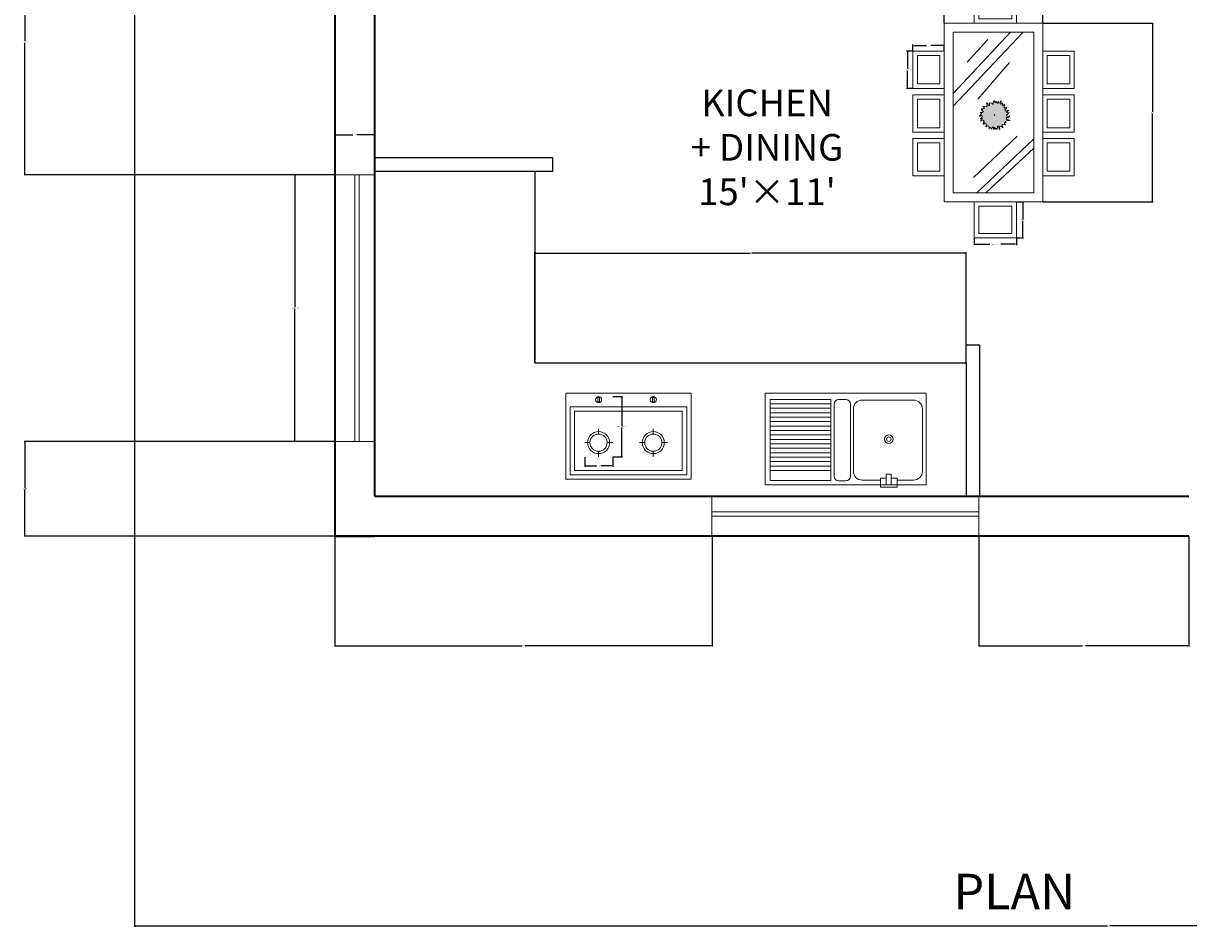
# Model space of a CAD drawing. Units: inches. Extents: x 1315 to 1802, y 1702 to 2202.
# Tile 1 of 4: x 1315 to 1577, y 1702 to 1906. Entities that reach past the tile are written whole.
import ezdxf

# ---------------------------------------------------------------- set-up
doc = ezdxf.new("R2010")
doc.units = ezdxf.units.IN
for name, color, linetype, lineweight in [('A-ANNO-DIMS', 2, 'Continuous', 18), ('A-ANNO-TEXT', 3, 'Continuous', 25), ('A-AREA-IDEN', 3, 'Continuous', 18), ('A-CASE', 7, 'Continuous', 25), ('A-EQPM', 3, 'Continuous', 18), ('A-FLOR-FIXT', 30, 'Continuous', 18), ('A-FLOR-FIXT-PATT', 30, 'Continuous', 13), ('A-FURN', 8, 'Continuous', 18), ('A-FURN-PATT', 9, 'Continuous', 13), ('A-GLAZ', 4, 'Continuous', 18), ('A-WALL', 7, 'Continuous', 35)]:
    doc.layers.add(name, color=color, linetype=linetype, lineweight=lineweight)
doc.styles.get("Standard").update_dxf_attribs({"font": 'times.ttf'})
doc.dimstyles.get("Standard").update_dxf_attribs({"dimtxt": 0.18, "dimasz": 0.18, "dimexe": 0.18, "dimexo": 0.0625, "dimgap": 0.09, "dimtad": 0, "dimtih": 1, "dimtoh": 1, "dimdec": 4, "dimzin": 0, "dimdsep": 46, "dimtxsty": 'Standard', "dimcen": 0.09, "dimadec": 0, "dimazin": 0, "dimtfac": 1, "dimtdec": 4, "dimtofl": 0, "dimtmove": 0, "dimatfit": 3, "dimfxl": 1, "dimtolj": 1, "dimtzin": 0, "dimarcsym": 0})

# ---------------------------------------------------------------- blocks, each defined once
blk = doc.blocks.new('*U2')
for points in [[(0, 60.64), (-3.051, 56.238), (-4.196, 52.815), (-5.34, 47.925), (-6.103, 45.969), (-11.062, 50.859), (-18.691, 52.326), (-20.98, 47.436), (-20.217, 43.524), (-20.598, 39.611), (-25.939, 43.035), (-27.846, 49.392), (-33.186, 52.326), (-30.516, 47.436), (-31.279, 43.035), (-30.135, 38.144), (-33.568, 35.21), (-40.815, 36.677), (-49.208, 38.144), (-46.919, 36.677), (-42.341, 31.787), (-42.341, 28.364), (-46.537, 27.386), (-55.692, 27.386), (-49.97, 22.006), (-54.548, 21.028), (-46.156, 14.671), (-51.496, 11.248), (-59.888, 11.248), (-55.692, 8.803), (-53.785, 5.38), (-57.218, 3.423), (-60.651, -1.467), (-61.033, -4.89), (-59.125, -3.423), (-54.548, -1.467), (-51.496, -4.401), (-53.022, -10.269), (-59.125, -15.16), (-49.208, -13.204), (-58.362, -24.451), (-48.445, -21.028), (-43.486, -22.495), (-43.104, -25.918), (-47.3, -31.298), (-43.104, -30.32), (-48.445, -39.611), (-38.527, -31.787), (-40.815, -36.188), (-32.423, -37.166), (-33.568, -43.523), (-35.475, -49.392), (-28.609, -44.99), (-23.65, -46.457), (-22.124, -51.837), (-21.743, -57.705), (-19.073, -52.326), (-15.639, -51.837), (-12.588, -58.683), (-11.062, -54.771), (-6.866, -49.392), (-6.866, -53.304), (-4.959, -48.414), (-1.907, -61.617), (-1.144, -51.348), (4.578, -59.172), (5.341, -54.282), (9.918, -56.727), (12.207, -60.639), (12.97, -47.925), (14.877, -44.501), (17.547, -47.436), (19.455, -52.815), (22.888, -60.639), (21.743, -49.392), (23.65, -46.457), (29.754, -47.925), (35.094, -52.326), (37.001, -53.793), (33.187, -46.457), (32.042, -41.567), (35.094, -39.122), (43.868, -40.589), (47.682, -42.056), (43.105, -36.188), (43.105, -33.743), (46.538, -31.298), (50.352, -32.765), (46.919, -26.407), (55.693, -22.495), (60.652, -22.984), (66.374, -22.006), (59.889, -20.05), (54.167, -18.094), (51.878, -15.649), (49.589, -12.225), (51.497, -10.269), (57.981, -9.78), (63.322, -7.335), (64.466, -2.934)], [(64.848, -2.934), (59.507, -5.379), (56.456, -4.401), (51.878, -2.445), (52.26, 0.978), (55.311, 3.912), (59.889, 5.869), (62.94, 11.248), (58.363, 10.27), (54.548, 10.27), (51.115, 11.248), (53.785, 15.649), (57.981, 18.094), (60.652, 19.561), (56.074, 19.561), (51.115, 17.605), (46.538, 19.072), (46.156, 22.496), (49.589, 27.386), (52.26, 34.721), (49.589, 33.743), (44.249, 30.32), (41.197, 32.276), (41.579, 37.655), (43.868, 42.546), (43.105, 46.947), (40.053, 44.013), (36.238, 40.589), (33.568, 42.057), (33.95, 45.969), (35.476, 52.815), (31.28, 49.392), (26.702, 46.947), (28.228, 50.859), (28.609, 61.129), (24.795, 54.282), (18.692, 50.859), (17.929, 57.706), (12.97, 50.859), (7.248, 57.706), (5.341, 53.304), (0, 60.64)]]:
    blk.add_lwpolyline(points)
blk.add_lwpolyline([(0.382, 1.956), (0, 0), (1.907, 0.489), (2.289, 1.467)], close=True)
blk = doc.blocks.new('SEFVFT')
for p, q in [((1768.59, 1985.26), (1777.59, 1985.26)), ((1768.59, 1925.26), (1768.59, 1985.26)), ((1768.59, 1985.26), (1773.09, 1985.26)), ((1773.09, 1985.26), (1773.09, 1925.26)), ((1774.09, 1925.26), (1774.09, 1985.26)), ((1777.59, 1985.26), (1777.59, 1925.26)), ((1777.59, 1925.26), (1768.59, 1925.26)), ((1773.09, 1925.26), (1774.09, 1925.26))]:
    blk.add_line(p, q)
blk = doc.blocks.new('CHAIR-DINING-SIDE')
for points in [[(0, 8.39), (7.03, 8.39), (7.03, 0), (0, 0)], [(1, 7.39), (6.03, 7.39), (6.03, 1), (1, 1)]]:
    blk.add_lwpolyline(points, close=True)
blk = doc.blocks.new('CHAIR-DINING-END')
for points in [[(0, 0), (9.48, 0), (9.48, 8.13), (0, 8.13)], [(1, 1), (8.48, 1), (8.48, 7.13), (1, 7.13)]]:
    blk.add_lwpolyline(points, close=True)
blk = doc.blocks.new('COOKTOP-BURNER-CONTROL')
for p, q in [((3.08, 5.13), (3.08, 6.3)), ((3.08, 6.3), (3.08, 5.13)), ((1.15, 3.2), (0, 3.2)), ((5.01, 3.2), (6.25, 3.2)), ((6.25, 3.2), (5.01, 3.2)), ((3.08, 1.27), (3.08, 0))]:
    blk.add_line(p, q)
blk.add_lwpolyline([(2.89, 12.39), (3.26, 12.39), (3.26, 13.37), (2.89, 13.37)], close=True)
for centre, radius in [((3.08, 12.88), 0.694), ((3.08, 3.2), 2.47), ((3.08, 3.2), 1.93)]:
    blk.add_circle(centre, radius)
blk = doc.blocks.new('*D12')
at = {"layer": 'A-ANNO-DIMS', "color": 0, "lineweight": -2, "transparency": 16777216}
for p, q in [((1384.53, 1871.52), (1375.41, 1871.52)), ((1375.59, 1871.34), (1375.59, 1841.7)), ((1375.59, 1811.7), (1375.59, 1841.34)), ((1384.53, 1811.52), (1375.41, 1811.52))]:
    blk.add_line(p, q, dxfattribs=at)
at = {"layer": 'A-ANNO-DIMS', "color": 0, "transparency": 16777216}
for points in [[(1375.56, 1871.34), (1375.62, 1871.34), (1375.59, 1871.52)], [(1375.56, 1811.7), (1375.62, 1811.7), (1375.59, 1811.52)]]:
    blk.add_solid(points, dxfattribs=at)
at = {"layer": 'Defpoints', "color": 0, "transparency": 16777216}
for p in [(1375.59, 1871.52), (1384.59, 1871.52), (1384.59, 1811.52)]:
    blk.add_point(p, dxfattribs=at)
at = {"layer": 'A-ANNO-DIMS', "color": 0, "transparency": 16777216, "insert": (1375.59, 1841.52), "char_height": 0.18, "attachment_point": 5}
blk.add_mtext('\\A1;WINDOW 60 TYP.', dxfattribs=at)
blk = doc.blocks.new('*D13')
at = {"layer": 'A-ANNO-DIMS', "color": 0, "lineweight": -2, "transparency": 16777216}
for p, q in [((1384.59, 1871.58), (1384.59, 1880.7)), ((1384.77, 1880.52), (1388.63, 1880.52)), ((1393.41, 1880.52), (1389.55, 1880.52)), ((1393.59, 1871.58), (1393.59, 1880.7))]:
    blk.add_line(p, q, dxfattribs=at)
at = {"layer": 'A-ANNO-DIMS', "color": 0, "transparency": 16777216}
for points in [[(1384.77, 1880.55), (1384.77, 1880.49), (1384.59, 1880.52)], [(1393.41, 1880.55), (1393.41, 1880.49), (1393.59, 1880.52)]]:
    blk.add_solid(points, dxfattribs=at)
at = {"layer": 'Defpoints', "color": 0, "transparency": 16777216}
for p in [(1393.59, 1880.52), (1384.59, 1871.52), (1393.59, 1871.52)]:
    blk.add_point(p, dxfattribs=at)
at = {"layer": 'A-ANNO-DIMS', "color": 0, "transparency": 16777216, "insert": (1389.09, 1880.52), "char_height": 0.18, "attachment_point": 5}
blk.add_mtext('\\A1;9 TYP.', dxfattribs=at)
blk = doc.blocks.new('*D18')
at = {"layer": 'A-ANNO-DIMS', "color": 0, "lineweight": -2, "transparency": 16777216}
for p, q in [((1514.54, 1899.33), (1513.16, 1899.33)), ((1513.34, 1899.15), (1513.34, 1895.32)), ((1513.34, 1891.12), (1513.34, 1894.95)), ((1514.54, 1890.94), (1513.16, 1890.94))]:
    blk.add_line(p, q, dxfattribs=at)
at = {"layer": 'A-ANNO-DIMS', "color": 0, "transparency": 16777216}
for points in [[(1513.31, 1899.15), (1513.37, 1899.15), (1513.34, 1899.33)], [(1513.31, 1891.12), (1513.37, 1891.12), (1513.34, 1890.94)]]:
    blk.add_solid(points, dxfattribs=at)
at = {"layer": 'Defpoints', "color": 0, "transparency": 16777216}
for p in [(1513.34, 1899.33), (1514.6, 1899.33), (1514.6, 1890.94)]:
    blk.add_point(p, dxfattribs=at)
at = {"layer": 'A-ANNO-DIMS', "color": 0, "transparency": 16777216, "insert": (1513.34, 1895.14), "char_height": 0.18, "attachment_point": 5}
blk.add_mtext('\\A1;SIDE CHAIR 8 TYP.', dxfattribs=at)
blk = doc.blocks.new('*D19')
at = {"layer": 'A-ANNO-DIMS', "color": 0, "lineweight": -2, "transparency": 16777216}
for p, q in [((1514.6, 1899.39), (1514.6, 1900.77)), ((1514.78, 1900.59), (1517.66, 1900.59)), ((1521.46, 1900.59), (1518.58, 1900.59)), ((1521.64, 1899.39), (1521.64, 1900.77))]:
    blk.add_line(p, q, dxfattribs=at)
at = {"layer": 'A-ANNO-DIMS', "color": 0, "transparency": 16777216}
for points in [[(1514.78, 1900.62), (1514.78, 1900.56), (1514.6, 1900.59)], [(1521.46, 1900.62), (1521.46, 1900.56), (1521.64, 1900.59)]]:
    blk.add_solid(points, dxfattribs=at)
at = {"layer": 'Defpoints', "color": 0, "transparency": 16777216}
for p in [(1521.64, 1900.59), (1514.6, 1899.33), (1521.64, 1899.33)]:
    blk.add_point(p, dxfattribs=at)
at = {"layer": 'A-ANNO-DIMS', "color": 0, "transparency": 16777216, "insert": (1518.12, 1900.59), "char_height": 0.18, "attachment_point": 5}
blk.add_mtext('\\A1;7 TYP.', dxfattribs=at)
blk = doc.blocks.new('*D20')
at = {"layer": 'A-ANNO-DIMS', "color": 0, "lineweight": -2, "transparency": 16777216}
for p, q in [((1528.38, 1857.23), (1528.38, 1855.69)), ((1528.56, 1855.87), (1531.91, 1855.87)), ((1537.68, 1855.87), (1534.34, 1855.87)), ((1537.86, 1857.23), (1537.86, 1855.69))]:
    blk.add_line(p, q, dxfattribs=at)
at = {"layer": 'A-ANNO-DIMS', "color": 0, "transparency": 16777216}
for points in [[(1528.56, 1855.9), (1528.56, 1855.84), (1528.38, 1855.87)], [(1537.68, 1855.9), (1537.68, 1855.84), (1537.86, 1855.87)]]:
    blk.add_solid(points, dxfattribs=at)
at = {"layer": 'Defpoints', "color": 0, "transparency": 16777216}
for p in [(1528.38, 1857.3), (1537.86, 1857.3), (1537.86, 1855.87)]:
    blk.add_point(p, dxfattribs=at)
at = {"layer": 'A-ANNO-DIMS', "color": 0, "transparency": 16777216, "insert": (1533.12, 1855.87), "char_height": 0.18, "attachment_point": 5}
blk.add_mtext('\\A1;END CHAIR 9 TYP.', dxfattribs=at)
blk = doc.blocks.new('*D21')
at = {"layer": 'A-ANNO-DIMS', "color": 0, "lineweight": -2, "transparency": 16777216}
for p, q in [((1537.92, 1865.42), (1539.46, 1865.42)), ((1539.28, 1865.24), (1539.28, 1861.54)), ((1539.28, 1857.48), (1539.28, 1861.18)), ((1537.92, 1857.3), (1539.46, 1857.3))]:
    blk.add_line(p, q, dxfattribs=at)
at = {"layer": 'A-ANNO-DIMS', "color": 0, "transparency": 16777216}
for points in [[(1539.25, 1865.24), (1539.31, 1865.24), (1539.28, 1865.42)], [(1539.25, 1857.48), (1539.31, 1857.48), (1539.28, 1857.3)]]:
    blk.add_solid(points, dxfattribs=at)
at = {"layer": 'Defpoints', "color": 0, "transparency": 16777216}
for p in [(1537.86, 1865.42), (1539.28, 1865.42), (1537.86, 1857.3)]:
    blk.add_point(p, dxfattribs=at)
at = {"layer": 'A-ANNO-DIMS', "color": 0, "transparency": 16777216, "insert": (1539.28, 1861.36), "char_height": 0.18, "attachment_point": 5}
blk.add_mtext('\\A1;8 TYP.', dxfattribs=at)
blk = doc.blocks.new('*D22')
at = {"layer": 'A-ANNO-DIMS', "color": 0, "lineweight": -2, "transparency": 16777216}
for p, q in [((1447.14, 1821.64), (1449.29, 1821.64)), ((1449.11, 1821.46), (1449.11, 1815.04)), ((1449.11, 1808.25), (1449.11, 1814.68)), ((1447.14, 1808.07), (1449.29, 1808.07))]:
    blk.add_line(p, q, dxfattribs=at)
at = {"layer": 'A-ANNO-DIMS', "color": 0, "transparency": 16777216}
for points in [[(1449.08, 1821.46), (1449.14, 1821.46), (1449.11, 1821.64)], [(1449.08, 1808.25), (1449.14, 1808.25), (1449.11, 1808.07)]]:
    blk.add_solid(points, dxfattribs=at)
at = {"layer": 'Defpoints', "color": 0, "transparency": 16777216}
for p in [(1447.08, 1821.64), (1449.11, 1821.64), (1447.08, 1808.07)]:
    blk.add_point(p, dxfattribs=at)
at = {"layer": 'A-ANNO-DIMS', "color": 0, "transparency": 16777216, "insert": (1449.11, 1814.86), "char_height": 0.18, "attachment_point": 5}
blk.add_mtext('\\A1;BURNER UNIT 14 TYP.', dxfattribs=at)
blk = doc.blocks.new('*D23')
at = {"layer": 'A-ANNO-DIMS', "color": 0, "lineweight": -2, "transparency": 16777216}
for p, q in [((1440.83, 1808.01), (1440.83, 1805.85)), ((1447.08, 1808.01), (1447.08, 1805.85)), ((1441.01, 1806.03), (1443.49, 1806.03)), ((1446.9, 1806.03), (1444.41, 1806.03))]:
    blk.add_line(p, q, dxfattribs=at)
at = {"layer": 'A-ANNO-DIMS', "color": 0, "transparency": 16777216}
for points in [[(1441.01, 1806.06), (1441.01, 1806), (1440.83, 1806.03)], [(1446.9, 1806.06), (1446.9, 1806), (1447.08, 1806.03)]]:
    blk.add_solid(points, dxfattribs=at)
at = {"layer": 'Defpoints', "color": 0, "transparency": 16777216}
for p in [(1440.83, 1808.07), (1447.08, 1808.07), (1447.08, 1806.03)]:
    blk.add_point(p, dxfattribs=at)
at = {"layer": 'A-ANNO-DIMS', "color": 0, "transparency": 16777216, "insert": (1443.95, 1806.03), "char_height": 0.18, "attachment_point": 5}
blk.add_mtext('\\A1;6 TYP.', dxfattribs=at)
blk = doc.blocks.new('*D28')
at = {"layer": 'A-ANNO-DIMS', "color": 0, "lineweight": -2, "transparency": 16777216}
for p, q in [((1339.59, 1931.18), (1339.59, 1702.41)), ((1777.59, 1763.18), (1777.59, 1702.41)), ((1339.77, 1702.59), (1558.31, 1702.59)), ((1777.41, 1702.59), (1558.87, 1702.59))]:
    blk.add_line(p, q, dxfattribs=at)
at = {"layer": 'A-ANNO-DIMS', "color": 0, "transparency": 16777216}
for points in [[(1339.77, 1702.62), (1339.77, 1702.56), (1339.59, 1702.59)], [(1777.41, 1702.62), (1777.41, 1702.56), (1777.59, 1702.59)]]:
    blk.add_solid(points, dxfattribs=at)
at = {"layer": 'Defpoints', "color": 0, "transparency": 16777216}
for p in [(1339.59, 1931.24), (1777.59, 1763.24), (1777.59, 1702.59)]:
    blk.add_point(p, dxfattribs=at)
at = {"layer": 'A-ANNO-DIMS', "color": 0, "transparency": 16777216, "insert": (1558.59, 1702.59), "char_height": 0.18, "attachment_point": 5}
blk.add_mtext('\\A1;438', dxfattribs=at)
blk = doc.blocks.new('*D39')
at = {"layer": 'A-ANNO-DIMS', "color": 0, "lineweight": -2, "transparency": 16777216}
for p, q in [((1384.53, 1931.24), (1314.76, 1931.24)), ((1314.94, 1931.06), (1314.94, 1901.56)), ((1314.94, 1871.7), (1314.94, 1901.2)), ((1384.53, 1871.52), (1314.76, 1871.52))]:
    blk.add_line(p, q, dxfattribs=at)
at = {"layer": 'A-ANNO-DIMS', "color": 0, "transparency": 16777216}
for points in [[(1314.91, 1931.06), (1314.97, 1931.06), (1314.94, 1931.24)], [(1314.91, 1871.7), (1314.97, 1871.7), (1314.94, 1871.52)]]:
    blk.add_solid(points, dxfattribs=at)
at = {"layer": 'Defpoints', "color": 0, "transparency": 16777216}
for p in [(1384.59, 1931.24), (1314.94, 1871.52), (1384.59, 1871.52)]:
    blk.add_point(p, dxfattribs=at)
at = {"layer": 'A-ANNO-DIMS', "color": 0, "transparency": 16777216, "insert": (1314.94, 1901.38), "char_height": 0.18, "attachment_point": 5}
blk.add_mtext('\\A1;59.72', dxfattribs=at)
blk = doc.blocks.new('*D40')
at = {"layer": 'A-ANNO-DIMS', "color": 0, "lineweight": -2, "transparency": 16777216}
for p, q in [((1384.53, 1811.52), (1314.76, 1811.52)), ((1314.94, 1811.34), (1314.94, 1801.06)), ((1314.94, 1790.42), (1314.94, 1800.7)), ((1384.53, 1790.24), (1314.76, 1790.24))]:
    blk.add_line(p, q, dxfattribs=at)
at = {"layer": 'A-ANNO-DIMS', "color": 0, "transparency": 16777216}
for points in [[(1314.91, 1811.34), (1314.97, 1811.34), (1314.94, 1811.52)], [(1314.91, 1790.42), (1314.97, 1790.42), (1314.94, 1790.24)]]:
    blk.add_solid(points, dxfattribs=at)
at = {"layer": 'Defpoints', "color": 0, "transparency": 16777216}
for p in [(1384.59, 1811.52), (1314.94, 1790.24), (1384.59, 1790.24)]:
    blk.add_point(p, dxfattribs=at)
at = {"layer": 'A-ANNO-DIMS', "color": 0, "transparency": 16777216, "insert": (1314.94, 1800.88), "char_height": 0.18, "attachment_point": 5}
blk.add_mtext('\\A1;21.276', dxfattribs=at)
blk = doc.blocks.new('*D45')
at = {"layer": 'A-ANNO-DIMS', "color": 0, "lineweight": -2, "transparency": 16777216}
for p, q in [((1384.59, 1790.18), (1384.59, 1765.41)), ((1469.41, 1790.18), (1469.41, 1765.41)), ((1384.77, 1765.59), (1426.62, 1765.59)), ((1469.23, 1765.59), (1427.37, 1765.59))]:
    blk.add_line(p, q, dxfattribs=at)
at = {"layer": 'A-ANNO-DIMS', "color": 0, "transparency": 16777216}
for points in [[(1384.77, 1765.62), (1384.77, 1765.56), (1384.59, 1765.59)], [(1469.23, 1765.62), (1469.23, 1765.56), (1469.41, 1765.59)]]:
    blk.add_solid(points, dxfattribs=at)
at = {"layer": 'Defpoints', "color": 0, "transparency": 16777216}
for p in [(1384.59, 1790.24), (1469.41, 1790.24), (1384.59, 1765.59)]:
    blk.add_point(p, dxfattribs=at)
at = {"layer": 'A-ANNO-DIMS', "color": 0, "transparency": 16777216, "insert": (1427, 1765.59), "char_height": 0.18, "attachment_point": 5}
blk.add_mtext('\\A1;84.82', dxfattribs=at)
blk = doc.blocks.new('*D46')
at = {"layer": 'A-ANNO-DIMS', "color": 0, "lineweight": -2, "transparency": 16777216}
for p, q in [((1529.41, 1790.18), (1529.41, 1765.41)), ((1576.59, 1790.18), (1576.59, 1765.41)), ((1529.59, 1765.59), (1552.62, 1765.59)), ((1576.41, 1765.59), (1553.38, 1765.59))]:
    blk.add_line(p, q, dxfattribs=at)
at = {"layer": 'A-ANNO-DIMS', "color": 0, "transparency": 16777216}
for points in [[(1529.59, 1765.62), (1529.59, 1765.56), (1529.41, 1765.59)], [(1576.41, 1765.62), (1576.41, 1765.56), (1576.59, 1765.59)]]:
    blk.add_solid(points, dxfattribs=at)
at = {"layer": 'Defpoints', "color": 0, "transparency": 16777216}
for p in [(1529.41, 1790.24), (1576.59, 1790.24), (1529.41, 1765.59)]:
    blk.add_point(p, dxfattribs=at)
at = {"layer": 'A-ANNO-DIMS', "color": 0, "transparency": 16777216, "insert": (1553, 1765.59), "char_height": 0.18, "attachment_point": 5}
blk.add_mtext('\\A1;47.18', dxfattribs=at)
blk = doc.blocks.new('*D55')
at = {"layer": 'A-ANNO-DIMS', "color": 0, "lineweight": -2, "transparency": 16777216}
for p, q in [((1521.64, 1905.63), (1521.64, 1930.4)), ((1521.82, 1930.22), (1532.27, 1930.22)), ((1543.62, 1930.22), (1533.17, 1930.22)), ((1543.8, 1905.63), (1543.8, 1930.4))]:
    blk.add_line(p, q, dxfattribs=at)
at = {"layer": 'A-ANNO-DIMS', "color": 0, "transparency": 16777216}
for points in [[(1521.82, 1930.25), (1521.82, 1930.19), (1521.64, 1930.22)], [(1543.62, 1930.25), (1543.62, 1930.19), (1543.8, 1930.22)]]:
    blk.add_solid(points, dxfattribs=at)
at = {"layer": 'Defpoints', "color": 0, "transparency": 16777216}
for p in [(1543.8, 1930.22), (1521.64, 1905.57), (1543.8, 1905.57)]:
    blk.add_point(p, dxfattribs=at)
at = {"layer": 'A-ANNO-DIMS', "color": 0, "transparency": 16777216, "insert": (1532.72, 1930.22), "char_height": 0.18, "attachment_point": 5}
blk.add_mtext('\\A1;22.164', dxfattribs=at)
blk = doc.blocks.new('*D56')
at = {"layer": 'A-ANNO-DIMS', "color": 0, "lineweight": -2, "transparency": 16777216}
for p, q in [((1543.86, 1905.57), (1568.63, 1905.57)), ((1568.45, 1905.39), (1568.45, 1885.68)), ((1568.45, 1865.6), (1568.45, 1885.31)), ((1543.86, 1865.42), (1568.63, 1865.42))]:
    blk.add_line(p, q, dxfattribs=at)
at = {"layer": 'A-ANNO-DIMS', "color": 0, "transparency": 16777216}
for points in [[(1568.42, 1905.39), (1568.48, 1905.39), (1568.45, 1905.57)], [(1568.42, 1865.6), (1568.48, 1865.6), (1568.45, 1865.42)]]:
    blk.add_solid(points, dxfattribs=at)
at = {"layer": 'Defpoints', "color": 0, "transparency": 16777216}
for p in [(1543.8, 1905.57), (1543.8, 1865.42), (1568.45, 1865.42)]:
    blk.add_point(p, dxfattribs=at)
at = {"layer": 'A-ANNO-DIMS', "color": 0, "transparency": 16777216, "insert": (1568.45, 1885.5), "char_height": 0.18, "attachment_point": 5}
blk.add_mtext('\\A1;40.146', dxfattribs=at)
blk = doc.blocks.new('*D57')
at = {"layer": 'A-ANNO-DIMS', "color": 0, "lineweight": -2, "transparency": 16777216}
for p, q in [((1429.59, 1829.3), (1429.59, 1854.07)), ((1429.77, 1853.89), (1477.88, 1853.89)), ((1526.41, 1853.89), (1478.3, 1853.89)), ((1526.59, 1829.3), (1526.59, 1854.07))]:
    blk.add_line(p, q, dxfattribs=at)
at = {"layer": 'A-ANNO-DIMS', "color": 0, "transparency": 16777216}
for points in [[(1429.77, 1853.92), (1429.77, 1853.86), (1429.59, 1853.89)], [(1526.41, 1853.92), (1526.41, 1853.86), (1526.59, 1853.89)]]:
    blk.add_solid(points, dxfattribs=at)
at = {"layer": 'Defpoints', "color": 0, "transparency": 16777216}
for p in [(1526.59, 1853.89), (1429.59, 1829.24), (1526.59, 1829.24)]:
    blk.add_point(p, dxfattribs=at)
at = {"layer": 'A-ANNO-DIMS', "color": 0, "transparency": 16777216, "insert": (1478.09, 1853.89), "char_height": 0.18, "attachment_point": 5}
blk.add_mtext('\\A1;97', dxfattribs=at)

msp = doc.modelspace()

# ---------------------------------------------------------------- hatches: boundary and pattern name
at = {"layer": 'A-FLOR-FIXT-PATT'}
h = msp.add_hatch(dxfattribs=at)
h.set_pattern_fill('ANSI31', color=256, scale=0.3149606, angle=-45, style=0)
h.paths.add_polyline_path([(1482.5042, 1804.5339), (1496.1497, 1804.5339), (1496.1497, 1820.4339), (1482.5042, 1820.4339)])
at = {"layer": 'A-FURN-PATT'}
h = msp.add_hatch(color=256, dxfattribs=at)
h.dxf.hatch_style = 1
h.paths.add_polyline_path([(1535.9712, 1884.3799), (1536.256, 1884.5103), (1536.3142, 1884.7343), (1536.0526, 1884.6145), (1535.8899, 1884.6667), (1535.6458, 1884.771), (1535.6662, 1884.9535), (1535.8289, 1885.1099), (1536.0729, 1885.2142), (1536.2356, 1885.501), (1535.9916, 1885.4489), (1535.7882, 1885.4489), (1535.6051, 1885.501), (1535.7475, 1885.7357), (1535.9712, 1885.866), (1536.1136, 1885.9443), (1535.8695, 1885.9443), (1535.6051, 1885.84), (1535.3611, 1885.9182), (1535.3407, 1886.1007), (1535.5238, 1886.3615), (1535.6662, 1886.7525), (1535.5238, 1886.7004), (1535.2391, 1886.5179), (1535.0763, 1886.6222), (1535.0967, 1886.909), (1535.2187, 1887.1697), (1535.1781, 1887.4044), (1535.0153, 1887.248), (1534.8119, 1887.0654), (1534.6696, 1887.1437), (1534.69, 1887.3522), (1534.7713, 1887.7173), (1534.5476, 1887.5347), (1534.3035, 1887.4044), (1534.3849, 1887.613), (1534.4052, 1888.1605), (1534.2018, 1887.7955), (1533.8764, 1887.613), (1533.8358, 1887.978), (1533.5714, 1887.613), (1533.2663, 1887.978), (1533.1646, 1887.7433), (1532.8798, 1888.1345), (1532.7172, 1887.8998), (1532.6561, 1887.7173), (1532.5951, 1887.4565), (1532.5545, 1887.3522), (1532.2901, 1887.613), (1531.8833, 1887.6912), (1531.7613, 1887.4305), (1531.8019, 1887.2219), (1531.7816, 1887.0133), (1531.4969, 1887.1958), (1531.3952, 1887.5347), (1531.1105, 1887.6912), (1531.2528, 1887.4305), (1531.2122, 1887.1958), (1531.2732, 1886.935), (1531.0901, 1886.7786), (1530.7037, 1886.8568), (1530.2562, 1886.935), (1530.3783, 1886.8568), (1530.6224, 1886.5961), (1530.6224, 1886.4136), (1530.3986, 1886.3615), (1529.9105, 1886.3615), (1530.2156, 1886.0746), (1529.9715, 1886.0225), (1530.419, 1885.6835), (1530.1343, 1885.501), (1529.6868, 1885.501), (1529.9105, 1885.3707), (1530.0122, 1885.1882), (1529.8292, 1885.0838), (1529.6461, 1884.8231), (1529.6258, 1884.6406), (1529.7275, 1884.7188), (1529.9715, 1884.8231), (1530.1343, 1884.6667), (1530.0529, 1884.3538), (1529.7275, 1884.093), (1530.2562, 1884.1973), (1529.7682, 1883.5977), (1530.2969, 1883.7802), (1530.5613, 1883.702), (1530.5817, 1883.5195), (1530.358, 1883.2326), (1530.5817, 1883.2848), (1530.2969, 1882.7894), (1530.8257, 1883.2066), (1530.7037, 1882.9719), (1531.1512, 1882.9198), (1531.0901, 1882.5808), (1530.9884, 1882.2679), (1531.3545, 1882.5026), (1531.6189, 1882.4244), (1531.7003, 1882.1375), (1531.7206, 1881.8247), (1531.8629, 1882.1115), (1532.046, 1882.1375), (1532.2087, 1881.7725), (1532.2901, 1881.9811), (1532.5138, 1882.2679), (1532.5138, 1882.0593), (1532.6155, 1882.3201), (1532.7782, 1881.6161), (1532.8189, 1882.1636), (1533.1239, 1881.7465), (1533.1646, 1882.0072), (1533.4086, 1881.8768), (1533.5307, 1881.6683), (1533.5714, 1882.3461), (1533.673, 1882.5287), (1533.8154, 1882.3722), (1533.9171, 1882.0854), (1534.1002, 1881.6683), (1534.0391, 1882.2679), (1534.1408, 1882.4244), (1534.4662, 1882.3461), (1534.7509, 1882.1115), (1534.8526, 1882.0333), (1534.6493, 1882.4244), (1534.5882, 1882.6851), (1534.7509, 1882.8155), (1535.2187, 1882.7373), (1535.4221, 1882.659), (1535.1781, 1882.9719), (1535.1781, 1883.1023), (1535.3611, 1883.2326), (1535.5645, 1883.1544), (1535.3814, 1883.4934), (1535.8492, 1883.702), (1536.1136, 1883.6759), (1536.4187, 1883.728), (1536.0729, 1883.8323), (1535.7679, 1883.9366), (1535.6458, 1884.067), (1535.5238, 1884.2495), (1535.6255, 1884.3538)])
h.paths.add_polyline_path([(1532.8798, 1884.9013), (1532.9002, 1885.0056), (1533.0019, 1884.9795), (1532.9815, 1884.9274)], flags=16)

# ---------------------------------------------------------------- linework, layer by layer
at = {"layer": 'A-CASE'}
for p, q in [((1433.5889, 1875.2999), (1393.5889, 1875.2999)), ((1433.5889, 1872.2999), (1433.5889, 1875.2999)), ((1393.5889, 1872.2999), (1429.5889, 1872.2999)), ((1429.5889, 1872.2999), (1429.5889, 1829.2411)), ((1429.5889, 1872.2999), (1433.5889, 1872.2999)), ((1526.5889, 1829.2411), (1526.5889, 1833.2411)), ((1526.5889, 1833.2411), (1529.5889, 1833.2411)), ((1529.5889, 1833.2411), (1529.5889, 1799.2411)), ((1429.5889, 1829.2411), (1526.5889, 1829.2411)), ((1526.5889, 1829.2411), (1526.5889, 1799.2411))]:
    msp.add_line(p, q, dxfattribs=at)
at = {"layer": 'A-EQPM'}
for points in [[(1464.7256, 1822.3821), (1436.5081, 1822.3821), (1436.5081, 1803.0157), (1464.7256, 1803.0157)], [(1463.7256, 1819.3085), (1437.5081, 1819.3085), (1437.5081, 1804.0157), (1463.7256, 1804.0157)], [(1462.7256, 1818.3085), (1438.5081, 1818.3085), (1438.5081, 1805.0157), (1462.7256, 1805.0157)]]:
    msp.add_lwpolyline(points, close=True, dxfattribs=at)
at = {"layer": 'A-FLOR-FIXT'}
msp.add_line((1482.5042, 1820.9839), (1482.5042, 1819.9839), dxfattribs=at)
for points in [[(1517.5286, 1801.7938), (1481.353, 1801.7938), (1481.353, 1822.3821), (1517.5286, 1822.3821)], [(1482.5042, 1802.7377), (1496.1497, 1802.7377), (1496.1497, 1820.9839), (1482.5042, 1820.9839)], [(1508.5947, 1801.7938), (1509.7235, 1801.7938), (1509.7235, 1804.1572), (1508.5947, 1804.1572)]]:
    msp.add_lwpolyline(points, close=True, dxfattribs=at)
msp.add_lwpolyline([(1497.8704, 1820.9359), (1499.522, 1820.9359, -0.41421356), (1500.522, 1819.9359), (1500.522, 1803.6897, -0.41421356), (1499.522, 1802.6897), (1497.8704, 1802.6897, -0.41421356), (1496.8704, 1803.6897), (1496.8704, 1819.9359, -0.41421356)], format="xyb", close=True, dxfattribs=at)
msp.add_lwpolyline([(1507.3073, 1802.8337), (1503.1947, 1802.8337, -0.41421356), (1501.1947, 1804.8337), (1501.1947, 1818.8399, -0.41421356), (1503.1947, 1820.8399), (1514.714, 1820.8399, -0.41421356), (1516.714, 1818.8399), (1516.714, 1804.8337, -0.41421356), (1514.714, 1802.8337), (1511.0053, 1802.8337)], format="xyb", dxfattribs=at)
msp.add_lwpolyline([(1508.5947, 1803.2408), (1507.3073, 1803.2408), (1507.3073, 1801.2577), (1511.0053, 1801.2577), (1511.0053, 1803.2408), (1509.7235, 1803.2408)], dxfattribs=at)
for radius in [0.9847, 0.5123]:
    msp.add_circle((1509.1591, 1812.04), radius, dxfattribs=at)
at = {"layer": 'A-FURN'}
for p, q in [((1523.6357, 1889.7782), (1536.5397, 1903.5683)), ((1539.3365, 1903.5683), (1523.6357, 1886.9056)), ((1536.5397, 1903.5683), (1539.3365, 1903.5683)), ((1526.7512, 1896.8431), (1531.4124, 1901.8895)), ((1529.1595, 1888.536), (1536.3067, 1896.7655)), ((1528.2272, 1870.9125), (1538.0158, 1880.1512)), ((1541.7995, 1879.6078), (1528.9264, 1867.4224)), ((1541.7995, 1877.5116), (1541.7995, 1879.6078)), ((1530.9463, 1867.4224), (1541.7995, 1877.5116))]:
    msp.add_line(p, q, dxfattribs=at)
for points in [[(1521.6357, 1905.5683), (1543.7995, 1905.5683), (1543.7995, 1865.4224), (1521.6357, 1865.4224)], [(1523.6357, 1903.5683), (1541.7995, 1903.5683), (1541.7995, 1867.4224), (1523.6357, 1867.4224)]]:
    msp.add_lwpolyline(points, close=True, dxfattribs=at)
at = {"layer": 'A-WALL'}
for p, q in [((1384.5889, 1931.2411), (1384.5889, 1790.2411)), ((1393.5889, 1799.2411), (1393.5889, 1931.2411)), ((1393.5889, 1799.2411), (1576.5889, 1799.2411)), ((1576.5889, 1790.2411), (1384.5889, 1790.2411)), ((1384.5889, 1790.2411), (1393.5889, 1790.2411))]:
    msp.add_line(p, q, dxfattribs=at)

# ---------------------------------------------------------------- block references
at = {"layer": 'A-EQPM'}
for p in [(1440.827, 1808.07), (1453.1356, 1808.07)]:
    msp.add_blockref('COOKTOP-BURNER-CONTROL', p, dxfattribs=at)
at = {"layer": 'A-FURN'}
for name, p in [('CHAIR-DINING-END', (1528.381, 1905.568)), ('CHAIR-DINING-SIDE', (1514.6011, 1890.944)), ('CHAIR-DINING-SIDE', (1543.8, 1890.944)), ('CHAIR-DINING-SIDE', (1514.6011, 1881.0841)), ('CHAIR-DINING-SIDE', (1543.8, 1881.0841)), ('CHAIR-DINING-SIDE', (1514.6011, 1871.3019)), ('CHAIR-DINING-SIDE', (1543.8, 1871.3019)), ('CHAIR-DINING-END', (1528.381, 1857.2955))]:
    msp.add_blockref(name, p, dxfattribs=at)
at = {"layer": 'A-FURN', "xscale": 0.0533167339335912, "yscale": 0.0533167339335912, "zscale": 0.0533167339335912}
msp.add_blockref('*U2', (1532.8798, 1884.9013), dxfattribs=at)
at = {"layer": 'A-GLAZ'}
msp.add_blockref('SEFVFT', (-384, -113.7386), dxfattribs=at)
at = {"layer": 'A-GLAZ', "rotation": 90}
msp.add_blockref('SEFVFT', (3454.6612, 21.6521), dxfattribs=at)

# ---------------------------------------------------------------- texts
at = {"layer": 'A-ANNO-TEXT', "insert": (1479.9708, 1714.3174), "char_height": 6, "attachment_point": 1}
msp.add_mtext_dynamic_manual_height_columns('\\pxqc;{\\H1.33333x;PLAN\\P\\H0.75x; }', width=114.825517, gutter_width=12.5, heights=[63.0068], dxfattribs=at)
at = {"layer": 'A-AREA-IDEN', "insert": (1424.3661, 1890.6786), "char_height": 6, "attachment_point": 1}
msp.add_mtext_dynamic_manual_height_columns("\\pxqc;{KICHEN\\P+ DINING\\P15'×11'}", width=114.825517, gutter_width=12.5, heights=[63.0068], dxfattribs=at)

# ---------------------------------------------------------------- dimensions: what is measured, and where the dimension line sits
at = {"layer": 'A-ANNO-DIMS'}
for base, p1, p2, angle, override, picture, middle in [((1314.9389, 1871.5173), (1384.5889, 1931.2411), (1384.5889, 1871.5173), 90, {"dimdec": 2, "dimlfac": 1, "dimrnd": 0, "dimzin": 0, "dimdsep": 46, "dimlunit": 2}, '*D39', (1314.9389, 1901.3792)), ((1568.4495, 1865.4224), (1543.7995, 1905.5683), (1543.7995, 1865.4224), 270, {"dimdec": 3, "dimlfac": 1, "dimrnd": 0, "dimzin": 0, "dimdsep": 46, "dimlunit": 2}, '*D56', (1568.4495, 1885.4954)), ((1314.9389, 1790.2411), (1384.5889, 1811.5173), (1384.5889, 1790.2411), 90, {"dimdec": 3, "dimlfac": 1, "dimrnd": 0, "dimzin": 0, "dimdsep": 46, "dimlunit": 2}, '*D40', (1314.9389, 1800.8792)), ((1384.5889, 1765.5911), (1469.4053, 1790.2411), (1384.5889, 1790.2411), 180, {"dimdec": 2, "dimlfac": 1, "dimrnd": 0, "dimzin": 0, "dimdsep": 46, "dimlunit": 2}, '*D45', (1426.9971, 1765.5911)), ((1529.4053, 1765.5911), (1576.5889, 1790.2411), (1529.4053, 1790.2411), 180, {"dimdec": 2, "dimlfac": 1, "dimrnd": 0, "dimzin": 0, "dimdsep": 46, "dimlunit": 2}, '*D46', (1552.9971, 1765.5911))]:
    dim = msp.add_linear_dim(base=base, p1=p1, p2=p2, angle=angle, dimstyle='Standard', override=override, dxfattribs=at)
    dim.commit()
    dim.dimension.update_dxf_attribs({"geometry": picture, "text_midpoint": middle})
for base, p1, p2, override, picture, middle in [((1777.5889, 1702.5911), (1339.5889, 1931.2411), (1777.5889, 1763.2411), {"dimdec": 0, "dimlfac": 1, "dimrnd": 0, "dimzin": 0, "dimdsep": 46, "dimlunit": 2}, '*D28', (1558.5889, 1702.5911)), ((1543.7995, 1930.2183), (1521.6357, 1905.5683), (1543.7995, 1905.5683), {"dimdec": 3, "dimlfac": 1, "dimrnd": 0, "dimzin": 0, "dimdsep": 46, "dimlunit": 2}, '*D55', (1532.7176, 1930.2183)), ((1526.5889, 1853.8911), (1429.5889, 1829.2411), (1526.5889, 1829.2411), {"dimdec": 0, "dimlfac": 1, "dimrnd": 0, "dimzin": 0, "dimdsep": 46, "dimlunit": 2}, '*D57', (1478.0889, 1853.8911))]:
    dim = msp.add_linear_dim(base=base, p1=p1, p2=p2, dimstyle='Standard', override=override, dxfattribs=at)
    dim.commit()
    dim.dimension.update_dxf_attribs({"geometry": picture, "text_midpoint": middle})
for base, p1, p2, text, picture, middle in [((1521.6357, 1900.5869), (1514.6007, 1899.3292), (1521.6357, 1899.3292), '<> TYP.', '*D19', (1518.1182, 1900.5869)), ((1393.5889, 1880.5173), (1384.5889, 1871.5173), (1393.5889, 1871.5173), '<> TYP.', '*D13', (1389.0889, 1880.5173)), ((1537.8591, 1855.8741), (1528.3813, 1857.2958), (1537.8591, 1857.2958), 'END CHAIR <> TYP.', '*D20', (1533.1202, 1855.8741)), ((1447.0752, 1806.0342), (1440.8274, 1808.0703), (1447.0752, 1808.0703), '<> TYP.', '*D23', (1443.9513, 1806.0342))]:
    dim = msp.add_linear_dim(base=base, p1=p1, p2=p2, text=text, dimstyle='Standard', override={"dimdec": 0, "dimlfac": 1, "dimrnd": 0, "dimzin": 0, "dimdsep": 46, "dimlunit": 2}, dxfattribs=at)
    dim.commit()
    dim.dimension.update_dxf_attribs({"geometry": picture, "text_midpoint": middle})
for base, p1, p2, text, picture, middle in [((1513.343, 1899.3292), (1514.6007, 1890.9444), (1514.6007, 1899.3292), 'SIDE CHAIR <> TYP.', '*D18', (1513.343, 1895.1368)), ((1375.5889, 1871.5173), (1384.5889, 1811.5173), (1384.5889, 1871.5173), 'WINDOW <> TYP.', '*D12', (1375.5889, 1841.5173)), ((1539.2808, 1865.4224), (1537.8591, 1857.2958), (1537.8591, 1865.4224), '<> TYP.', '*D21', (1539.2808, 1861.3591)), ((1449.1113, 1821.6442), (1447.0752, 1808.0703), (1447.0752, 1821.6442), 'BURNER UNIT <> TYP.', '*D22', (1449.1113, 1814.8572))]:
    dim = msp.add_linear_dim(base=base, p1=p1, p2=p2, angle=90, text=text, dimstyle='Standard', override={"dimdec": 0, "dimlfac": 1, "dimrnd": 0, "dimzin": 0, "dimdsep": 46, "dimlunit": 2}, dxfattribs=at)
    dim.commit()
    dim.dimension.update_dxf_attribs({"geometry": picture, "text_midpoint": middle})

doc.saveas('drawing.dxf')
